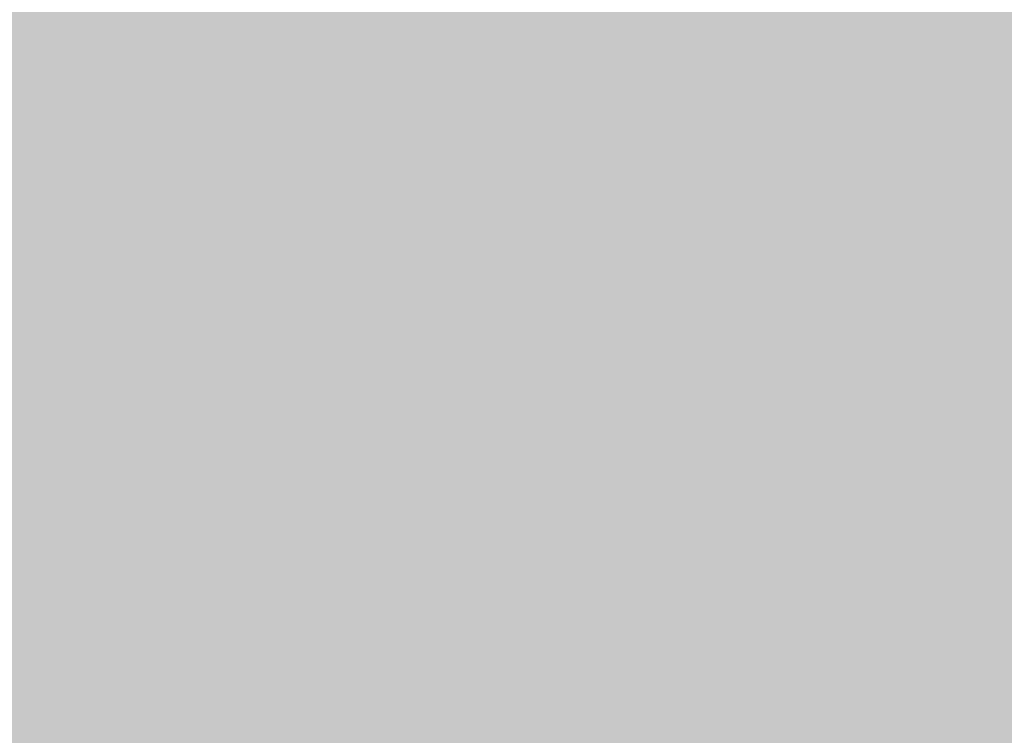
# Model space of a CAD drawing. Units: feet. Extents: x 3168 to 4724, y 827 to 1477.
# Tile 49 of 256: x 3273.072 to 3275.224, y 1096.781 to 1098.344. Entities that reach past the tile are written whole.
import ezdxf

# ---------------------------------------------------------------- set-up
doc = ezdxf.new("R2010")
doc.units = ezdxf.units.FT
doc.layers.add('A-ELEV-PATT', color=8, linetype='Continuous', lineweight=13)

msp = doc.modelspace()

# ---------------------------------------------------------------- hatches: boundary and pattern name
at = {"layer": 'A-ELEV-PATT'}
h = msp.add_hatch(color=256, dxfattribs=at)
h.dxf.hatch_style = 1
edge = h.paths.add_edge_path()
edge.add_ellipse((3552.9058, 979.2201), major_axis=(36.7449, 0), ratio=0.4848485, start_angle=0, end_angle=360)
edge = h.paths.add_edge_path()
edge.add_ellipse((3559.8916, 929.2523), major_axis=(36.7449, 0), ratio=0.4848485, start_angle=0, end_angle=360)
edge = h.paths.add_edge_path()
edge.add_line((3299.3168, 1198.6061), (3479.9167, 1198.6061))
edge.add_line((3479.9167, 1198.6061), (3479.9167, 1209.8686))
edge.add_spline(control_points=[(3479.9167, 1209.8686), (3464.3012, 1209.8686), (3448.6856, 1209.8686), (3410.9491, 1209.8686), (3388.8282, 1209.8686), (3355.6469, 1209.8686), (3344.5864, 1209.8686), (3327.9957, 1209.8686), (3322.4655, 1209.8686), (3314.1702, 1209.8686), (3311.4051, 1209.8686), (3307.2574, 1209.8686), (3305.8748, 1209.8686), (3303.801, 1209.8686), (3303.1097, 1209.8686), (3302.0728, 1209.8686), (3301.7272, 1209.8686), (3301.2087, 1209.8686), (3301.0359, 1209.8686), (3300.7767, 1209.8686), (3300.6903, 1209.8686), (3300.5606, 1209.8686), (3300.5174, 1209.8686), (3300.4526, 1209.8686), (3300.431, 1209.8686), (3300.3986, 1209.8686), (3300.3878, 1209.8686), (3300.3662, 1209.8686), (3300.3457, 1209.8686), (3300.3455, 1209.8686), (3300.3455, 1209.8686), (3300.3433, 1209.8686), (3300.3411, 1209.8686), (3300.3379, 1209.8686), (3300.3368, 1209.8686), (3300.3339, 1209.8686), (3300.3321, 1209.8686), (3300.3255, 1209.8686), (3300.3207, 1209.8686), (3300.3109, 1209.8686), (3300.306, 1209.8686), (3300.2905, 1209.8686), (3300.28, 1209.8686), (3300.2324, 1209.8688), (3300.1953, 1209.869), (3299.9511, 1209.8706), (3299.7448, 1209.8743), (3299.4368, 1209.8833), (3299.3344, 1209.8868), (3299.1811, 1209.8929), (3299.13, 1209.8951), (3298.6522, 1209.9168), (3298.2295, 1209.9457), (3297.6016, 1210.0024), (3297.3934, 1210.0235), (3297.0827, 1210.0583), (3296.9793, 1210.0705), (3296.293, 1210.1549), (3295.7181, 1210.2434), (3294.8687, 1210.3989), (3294.5877, 1210.4545), (3294.1693, 1210.5433), (3294.0304, 1210.5739), (3291.7071, 1211.1012), (3289.6536, 1211.8134), (3285.7763, 1213.564), (3283.9514, 1214.6035), (3280.5122, 1216.9801), (3278.8972, 1218.3176), (3276.3799, 1220.8295), (3275.416, 1221.9177), (3274.0393, 1223.7077), (3273.581, 1224.3495), (3273.1432, 1225.0163)], knot_values=[39.119033, 39.119033, 39.119033, 39.119033, 39.286353, 39.286353, 39.523379, 39.523379, 39.641892, 39.641892, 39.701148, 39.701148, 39.730777, 39.730777, 39.745591, 39.745591, 39.752998, 39.752998, 39.756701, 39.756701, 39.758553, 39.758553, 39.759479, 39.759479, 39.759942, 39.759942, 39.760173, 39.760173, 39.760289, 39.760289, 39.760405, 39.760405, 39.760463, 39.760463, 39.763389, 39.763389, 39.764851, 39.764851, 39.767304, 39.767304, 39.773825, 39.773825, 39.78057, 39.78057, 39.79477, 39.79477, 39.845194, 39.845194, 40.126715, 40.126715, 40.267476, 40.267476, 40.337856, 40.337856, 40.927023, 40.927023, 41.221606, 41.221606, 41.368898, 41.368898, 42.202622, 42.202622, 42.619485, 42.619485, 42.827916, 42.827916, 46.118323, 46.118323, 49.408731, 49.408731, 52.699139, 52.699139, 54.927489, 54.927489, 56.104228, 56.104228, 56.104228, 56.104228], weights=[1, 1, 1, 1, 1, 1, 1, 1, 1, 1, 1, 1, 1, 1, 1, 1, 1, 1, 1, 1, 1, 1, 1, 1, 1, 1, 1, 1, 1, 1, 1, 1, 1, 1, 1, 1, 1, 1, 1, 1, 1, 1, 1, 1, 1, 1, 1, 1, 1, 1, 1, 1, 1, 1, 1, 1, 1, 1, 1, 1, 1, 1, 1, 1, 1, 1, 1, 1, 1, 1, 1, 1, 1, 1], degree=3, periodic=0)
edge.add_line((3273.1432, 1225.0163), (3273.1432, 1099.0163))
edge.add_line((3273.1432, 1099.0163), (3299.3168, 1099.0163))
edge.add_line((3299.3168, 1099.0163), (3299.3168, 1198.6061))
edge = h.paths.add_edge_path()
edge.add_line((3304.7584, 1324.1581), (3479.9167, 1324.1581))
edge.add_line((3479.9167, 1324.1581), (3479.9167, 1335.7146))
edge.add_line((3479.9167, 1335.7146), (3269.1616, 1335.7146))
edge.add_spline(control_points=[(3269.1616, 1335.7146), (3264.0242, 1335.7146), (3258.3641, 1328.9582), (3259.2643, 1323.9003)], knot_values=[0, 0, 0, 0, 15.412191, 15.412191, 15.412191, 15.412191], degree=3, periodic=0)
edge.add_line((3259.2643, 1323.9003), (3265.5168, 1288.7691))
edge.add_line((3265.5168, 1288.7691), (3275.2651, 1261.5456))
edge.add_line((3275.2651, 1261.5456), (3304.7584, 1261.5456))
edge.add_line((3304.7584, 1261.5456), (3304.7584, 1324.1581))
h = msp.add_hatch(color=256, dxfattribs=at)
h.dxf.hatch_style = 1
h.paths.add_polyline_path([(3384.5252, 1099.0163), (3335.0292, 1099.0163), (3299.3168, 1099.0163), (3273.1432, 1099.0163), (3217.5654, 1099.0163), (3168.0693, 827.1163), (3335.0292, 827.1163)])

doc.saveas('drawing.dxf')
